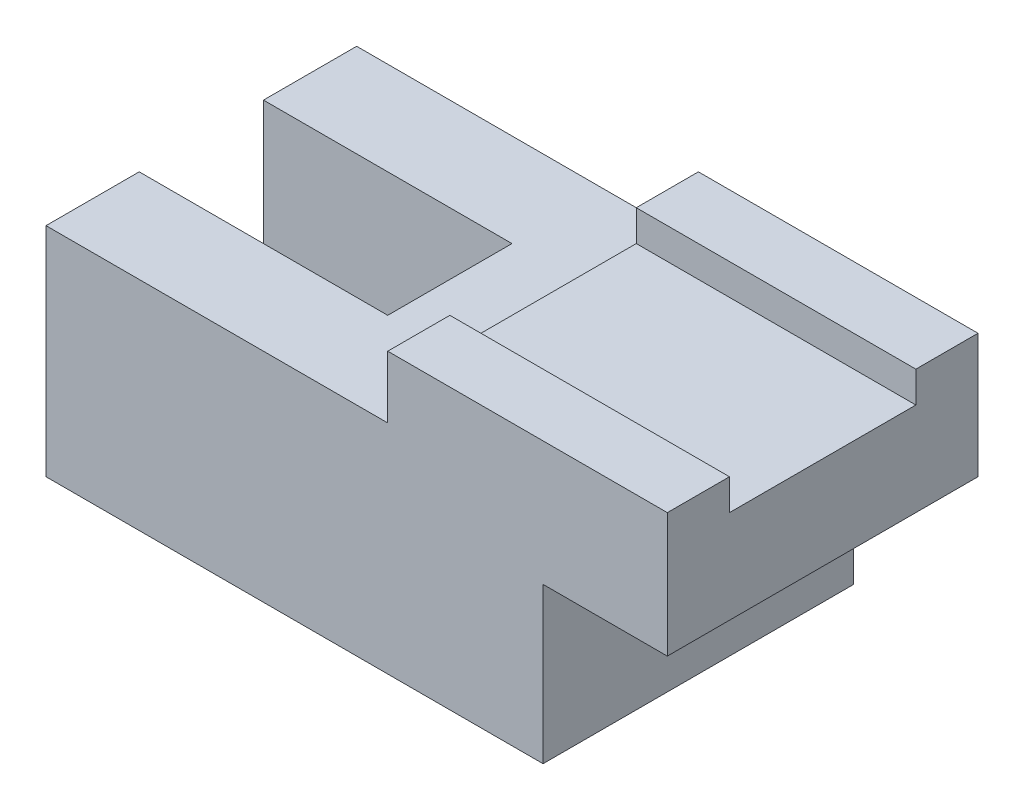
ISO-10303-21;
HEADER;
FILE_DESCRIPTION(('STEP AP214'),'2;1');
FILE_NAME('part.step','',(''),(''),'','','');
FILE_SCHEMA(('AUTOMOTIVE_DESIGN { 1 0 10303 214 1 1 1 1 }'));
ENDSEC;
DATA;
#1=APPLICATION_CONTEXT('core data for automotive mechanical design processes');
#2=APPLICATION_PROTOCOL_DEFINITION('international standard','automotive_design',2000,#1);
#3=PRODUCT_CONTEXT('',#1,'mechanical');
#4=PRODUCT('Part','Part','',(#3));
#5=PRODUCT_RELATED_PRODUCT_CATEGORY('part','',(#4));
#6=PRODUCT_DEFINITION_FORMATION('','',#4);
#7=PRODUCT_DEFINITION_CONTEXT('part definition',#1,'design');
#8=PRODUCT_DEFINITION('design','',#6,#7);
#9=PRODUCT_DEFINITION_SHAPE('','',#8);
#10=(LENGTH_UNIT() NAMED_UNIT(*) SI_UNIT(.MILLI.,.METRE.));
#11=(NAMED_UNIT(*) PLANE_ANGLE_UNIT() SI_UNIT($,.RADIAN.));
#12=(NAMED_UNIT(*) SI_UNIT($,.STERADIAN.) SOLID_ANGLE_UNIT());
#13=UNCERTAINTY_MEASURE_WITH_UNIT(LENGTH_MEASURE(1.E-05),#10,'distance_accuracy_value','');
#14=(GEOMETRIC_REPRESENTATION_CONTEXT(3) GLOBAL_UNCERTAINTY_ASSIGNED_CONTEXT((#13)) GLOBAL_UNIT_ASSIGNED_CONTEXT((#10,
#11,#12)) REPRESENTATION_CONTEXT('',''));
#15=CARTESIAN_POINT('',(0.,0.,0.));
#16=DIRECTION('',(0.,0.,1.));
#17=DIRECTION('',(1.,0.,0.));
#18=AXIS2_PLACEMENT_3D('',#15,#16,#17);
#19=CARTESIAN_POINT('',(100.,45.,50.));
#20=DIRECTION('',(0.,-1.,0.));
#21=DIRECTION('',(1.,0.,0.));
#22=AXIS2_PLACEMENT_3D('',#19,#20,#21);
#23=PLANE('',#22);
#24=DIRECTION('',(0.,0.,-1.));
#25=VECTOR('',#24,1.);
#26=CARTESIAN_POINT('',(100.,45.,50.));
#27=LINE('',#26,#25);
#28=CARTESIAN_POINT('',(100.,45.,50.));
#29=VERTEX_POINT('',#28);
#30=CARTESIAN_POINT('',(100.,45.,40.));
#31=VERTEX_POINT('',#30);
#32=EDGE_CURVE('E171',#29,#31,#27,.T.);
#33=ORIENTED_EDGE('',*,*,#32,.T.);
#34=DIRECTION('',(-1.,0.,0.));
#35=VECTOR('',#34,1.);
#36=CARTESIAN_POINT('',(100.,45.,40.));
#37=LINE('',#36,#35);
#38=CARTESIAN_POINT('',(55.,45.,40.));
#39=VERTEX_POINT('',#38);
#40=EDGE_CURVE('E279',#31,#39,#37,.T.);
#41=ORIENTED_EDGE('',*,*,#40,.T.);
#42=DIRECTION('',(0.,0.,-1.));
#43=VECTOR('',#42,1.);
#44=CARTESIAN_POINT('',(55.,45.,50.));
#45=LINE('',#44,#43);
#46=CARTESIAN_POINT('',(55.,45.,50.));
#47=VERTEX_POINT('',#46);
#48=EDGE_CURVE('E178',#47,#39,#45,.T.);
#49=ORIENTED_EDGE('',*,*,#48,.F.);
#50=DIRECTION('',(-1.,0.,0.));
#51=VECTOR('',#50,1.);
#52=CARTESIAN_POINT('',(100.,45.,50.));
#53=LINE('',#52,#51);
#54=EDGE_CURVE('E251',#29,#47,#53,.T.);
#55=ORIENTED_EDGE('',*,*,#54,.F.);
#56=EDGE_LOOP('',(#33,#41,#49,#55));
#57=FACE_BOUND('',#56,.T.);
#58=ADVANCED_FACE('F39',(#57),#23,.F.);
#59=CARTESIAN_POINT('',(0.,35.,50.));
#60=DIRECTION('',(1.,0.,0.));
#61=DIRECTION('',(0.,0.,-1.));
#62=AXIS2_PLACEMENT_3D('',#59,#60,#61);
#63=PLANE('',#62);
#64=DIRECTION('',(0.,0.,-1.));
#65=VECTOR('',#64,1.);
#66=CARTESIAN_POINT('',(0.,0.,50.));
#67=LINE('',#66,#65);
#68=CARTESIAN_POINT('',(0.,0.,15.));
#69=VERTEX_POINT('',#68);
#70=CARTESIAN_POINT('',(0.,0.,0.));
#71=VERTEX_POINT('',#70);
#72=EDGE_CURVE('E50',#69,#71,#67,.T.);
#73=ORIENTED_EDGE('',*,*,#72,.F.);
#74=DIRECTION('',(0.,-1.,0.));
#75=VECTOR('',#74,1.);
#76=CARTESIAN_POINT('',(0.,0.,15.));
#77=LINE('',#76,#75);
#78=CARTESIAN_POINT('',(0.,35.,15.));
#79=VERTEX_POINT('',#78);
#80=EDGE_CURVE('E272',#79,#69,#77,.T.);
#81=ORIENTED_EDGE('',*,*,#80,.F.);
#82=DIRECTION('',(0.,0.,-1.));
#83=VECTOR('',#82,1.);
#84=CARTESIAN_POINT('',(0.,35.,50.));
#85=LINE('',#84,#83);
#86=CARTESIAN_POINT('',(0.,35.,0.));
#87=VERTEX_POINT('',#86);
#88=EDGE_CURVE('E212',#79,#87,#85,.T.);
#89=ORIENTED_EDGE('',*,*,#88,.T.);
#90=DIRECTION('',(0.,-1.,0.));
#91=VECTOR('',#90,1.);
#92=CARTESIAN_POINT('',(0.,35.,0.));
#93=LINE('',#92,#91);
#94=EDGE_CURVE('E208',#87,#71,#93,.T.);
#95=ORIENTED_EDGE('',*,*,#94,.T.);
#96=EDGE_LOOP('',(#73,#81,#89,#95));
#97=FACE_BOUND('',#96,.T.);
#98=ADVANCED_FACE('F215',(#97),#63,.F.);
#99=CARTESIAN_POINT('',(0.,35.,50.));
#100=VERTEX_POINT('',#99);
#101=CARTESIAN_POINT('',(0.,35.,35.));
#102=VERTEX_POINT('',#101);
#103=EDGE_CURVE('E234',#100,#102,#85,.T.);
#104=ORIENTED_EDGE('',*,*,#103,.T.);
#105=DIRECTION('',(0.,1.,0.));
#106=VECTOR('',#105,1.);
#107=CARTESIAN_POINT('',(0.,35.,35.));
#108=LINE('',#107,#106);
#109=CARTESIAN_POINT('',(0.,0.,35.));
#110=VERTEX_POINT('',#109);
#111=EDGE_CURVE('E277',#110,#102,#108,.T.);
#112=ORIENTED_EDGE('',*,*,#111,.F.);
#113=CARTESIAN_POINT('',(0.,0.,50.));
#114=VERTEX_POINT('',#113);
#115=EDGE_CURVE('E11',#114,#110,#67,.T.);
#116=ORIENTED_EDGE('',*,*,#115,.F.);
#117=DIRECTION('',(0.,-1.,0.));
#118=VECTOR('',#117,1.);
#119=CARTESIAN_POINT('',(0.,35.,50.));
#120=LINE('',#119,#118);
#121=EDGE_CURVE('E231',#100,#114,#120,.T.);
#122=ORIENTED_EDGE('',*,*,#121,.F.);
#123=EDGE_LOOP('',(#104,#112,#116,#122));
#124=FACE_BOUND('',#123,.T.);
#125=ADVANCED_FACE('F41',(#124),#63,.F.);
#126=CARTESIAN_POINT('',(0.,0.,50.));
#127=DIRECTION('',(0.,1.,0.));
#128=DIRECTION('',(0.,0.,1.));
#129=AXIS2_PLACEMENT_3D('',#126,#127,#128);
#130=PLANE('',#129);
#131=DIRECTION('',(0.,0.,1.));
#132=VECTOR('',#131,1.);
#133=CARTESIAN_POINT('',(40.,0.,35.));
#134=LINE('',#133,#132);
#135=CARTESIAN_POINT('',(40.,0.,15.));
#136=VERTEX_POINT('',#135);
#137=CARTESIAN_POINT('',(40.,0.,35.));
#138=VERTEX_POINT('',#137);
#139=EDGE_CURVE('E274',#136,#138,#134,.T.);
#140=ORIENTED_EDGE('',*,*,#139,.F.);
#141=DIRECTION('',(-1.,0.,0.));
#142=VECTOR('',#141,1.);
#143=CARTESIAN_POINT('',(40.,0.,15.));
#144=LINE('',#143,#142);
#145=EDGE_CURVE('E199',#136,#69,#144,.T.);
#146=ORIENTED_EDGE('',*,*,#145,.T.);
#147=ORIENTED_EDGE('',*,*,#72,.T.);
#148=DIRECTION('',(1.,0.,0.));
#149=VECTOR('',#148,1.);
#150=CARTESIAN_POINT('',(0.,0.,0.));
#151=LINE('',#150,#149);
#152=CARTESIAN_POINT('',(80.,0.,0.));
#153=VERTEX_POINT('',#152);
#154=EDGE_CURVE('E200',#71,#153,#151,.T.);
#155=ORIENTED_EDGE('',*,*,#154,.T.);
#156=DIRECTION('',(0.,0.,-1.));
#157=VECTOR('',#156,1.);
#158=CARTESIAN_POINT('',(80.,0.,50.));
#159=LINE('',#158,#157);
#160=CARTESIAN_POINT('',(80.,0.,50.));
#161=VERTEX_POINT('',#160);
#162=EDGE_CURVE('E189',#161,#153,#159,.T.);
#163=ORIENTED_EDGE('',*,*,#162,.F.);
#164=DIRECTION('',(1.,0.,0.));
#165=VECTOR('',#164,1.);
#166=CARTESIAN_POINT('',(0.,0.,50.));
#167=LINE('',#166,#165);
#168=EDGE_CURVE('E263',#114,#161,#167,.T.);
#169=ORIENTED_EDGE('',*,*,#168,.F.);
#170=ORIENTED_EDGE('',*,*,#115,.T.);
#171=DIRECTION('',(-1.,0.,0.));
#172=VECTOR('',#171,1.);
#173=CARTESIAN_POINT('',(40.,0.,35.));
#174=LINE('',#173,#172);
#175=EDGE_CURVE('E266',#138,#110,#174,.T.);
#176=ORIENTED_EDGE('',*,*,#175,.F.);
#177=EDGE_LOOP('',(#140,#146,#147,#155,#163,#169,#170,#176));
#178=FACE_BOUND('',#177,.T.);
#179=ADVANCED_FACE('F196',(#178),#130,.F.);
#180=CARTESIAN_POINT('',(80.,0.,50.));
#181=DIRECTION('',(-1.,0.,0.));
#182=DIRECTION('',(0.,0.,1.));
#183=AXIS2_PLACEMENT_3D('',#180,#181,#182);
#184=PLANE('',#183);
#185=DIRECTION('',(0.,1.,0.));
#186=VECTOR('',#185,1.);
#187=CARTESIAN_POINT('',(80.,0.,0.));
#188=LINE('',#187,#186);
#189=CARTESIAN_POINT('',(80.,25.,0.));
#190=VERTEX_POINT('',#189);
#191=EDGE_CURVE('E209',#153,#190,#188,.T.);
#192=ORIENTED_EDGE('',*,*,#191,.T.);
#193=DIRECTION('',(0.,0.,-1.));
#194=VECTOR('',#193,1.);
#195=CARTESIAN_POINT('',(80.,25.,50.));
#196=LINE('',#195,#194);
#197=CARTESIAN_POINT('',(80.,25.,50.));
#198=VERTEX_POINT('',#197);
#199=EDGE_CURVE('E183',#198,#190,#196,.T.);
#200=ORIENTED_EDGE('',*,*,#199,.F.);
#201=DIRECTION('',(0.,1.,0.));
#202=VECTOR('',#201,1.);
#203=CARTESIAN_POINT('',(80.,0.,50.));
#204=LINE('',#203,#202);
#205=EDGE_CURVE('E261',#161,#198,#204,.T.);
#206=ORIENTED_EDGE('',*,*,#205,.F.);
#207=ORIENTED_EDGE('',*,*,#162,.T.);
#208=EDGE_LOOP('',(#192,#200,#206,#207));
#209=FACE_BOUND('',#208,.T.);
#210=ADVANCED_FACE('F311',(#209),#184,.F.);
#211=CARTESIAN_POINT('',(80.,25.,50.));
#212=DIRECTION('',(0.,1.,0.));
#213=DIRECTION('',(0.,0.,1.));
#214=AXIS2_PLACEMENT_3D('',#211,#212,#213);
#215=PLANE('',#214);
#216=DIRECTION('',(1.,0.,0.));
#217=VECTOR('',#216,1.);
#218=CARTESIAN_POINT('',(80.,25.,0.));
#219=LINE('',#218,#217);
#220=CARTESIAN_POINT('',(100.,25.,0.));
#221=VERTEX_POINT('',#220);
#222=EDGE_CURVE('E221',#190,#221,#219,.T.);
#223=ORIENTED_EDGE('',*,*,#222,.T.);
#224=DIRECTION('',(0.,0.,-1.));
#225=VECTOR('',#224,1.);
#226=CARTESIAN_POINT('',(100.,25.,50.));
#227=LINE('',#226,#225);
#228=CARTESIAN_POINT('',(100.,25.,50.));
#229=VERTEX_POINT('',#228);
#230=EDGE_CURVE('E179',#229,#221,#227,.T.);
#231=ORIENTED_EDGE('',*,*,#230,.F.);
#232=DIRECTION('',(1.,0.,0.));
#233=VECTOR('',#232,1.);
#234=CARTESIAN_POINT('',(80.,25.,50.));
#235=LINE('',#234,#233);
#236=EDGE_CURVE('E259',#198,#229,#235,.T.);
#237=ORIENTED_EDGE('',*,*,#236,.F.);
#238=ORIENTED_EDGE('',*,*,#199,.T.);
#239=EDGE_LOOP('',(#223,#231,#237,#238));
#240=FACE_BOUND('',#239,.T.);
#241=ADVANCED_FACE('F320',(#240),#215,.F.);
#242=CARTESIAN_POINT('',(100.,25.,50.));
#243=DIRECTION('',(-1.,0.,0.));
#244=DIRECTION('',(0.,0.,1.));
#245=AXIS2_PLACEMENT_3D('',#242,#243,#244);
#246=PLANE('',#245);
#247=DIRECTION('',(0.,0.,1.));
#248=VECTOR('',#247,1.);
#249=CARTESIAN_POINT('',(100.,40.,10.));
#250=LINE('',#249,#248);
#251=CARTESIAN_POINT('',(100.,40.,10.));
#252=VERTEX_POINT('',#251);
#253=CARTESIAN_POINT('',(100.,40.,40.));
#254=VERTEX_POINT('',#253);
#255=EDGE_CURVE('E158',#252,#254,#250,.T.);
#256=ORIENTED_EDGE('',*,*,#255,.T.);
#257=DIRECTION('',(0.,1.,0.));
#258=VECTOR('',#257,1.);
#259=CARTESIAN_POINT('',(100.,40.,40.));
#260=LINE('',#259,#258);
#261=EDGE_CURVE('E169',#254,#31,#260,.T.);
#262=ORIENTED_EDGE('',*,*,#261,.T.);
#263=ORIENTED_EDGE('',*,*,#32,.F.);
#264=DIRECTION('',(0.,1.,0.));
#265=VECTOR('',#264,1.);
#266=CARTESIAN_POINT('',(100.,25.,50.));
#267=LINE('',#266,#265);
#268=EDGE_CURVE('E254',#229,#29,#267,.T.);
#269=ORIENTED_EDGE('',*,*,#268,.F.);
#270=ORIENTED_EDGE('',*,*,#230,.T.);
#271=DIRECTION('',(0.,1.,0.));
#272=VECTOR('',#271,1.);
#273=CARTESIAN_POINT('',(100.,25.,0.));
#274=LINE('',#273,#272);
#275=CARTESIAN_POINT('',(100.,45.,0.));
#276=VERTEX_POINT('',#275);
#277=EDGE_CURVE('E172',#221,#276,#274,.T.);
#278=ORIENTED_EDGE('',*,*,#277,.T.);
#279=CARTESIAN_POINT('',(100.,45.,10.));
#280=VERTEX_POINT('',#279);
#281=EDGE_CURVE('E164',#280,#276,#27,.T.);
#282=ORIENTED_EDGE('',*,*,#281,.F.);
#283=DIRECTION('',(0.,-1.,0.));
#284=VECTOR('',#283,1.);
#285=CARTESIAN_POINT('',(100.,45.,10.));
#286=LINE('',#285,#284);
#287=EDGE_CURVE('E151',#280,#252,#286,.T.);
#288=ORIENTED_EDGE('',*,*,#287,.T.);
#289=EDGE_LOOP('',(#256,#262,#263,#269,#270,#278,#282,#288));
#290=FACE_BOUND('',#289,.T.);
#291=ADVANCED_FACE('F168',(#290),#246,.F.);
#292=CARTESIAN_POINT('',(55.,45.,10.));
#293=VERTEX_POINT('',#292);
#294=CARTESIAN_POINT('',(55.,45.,0.));
#295=VERTEX_POINT('',#294);
#296=EDGE_CURVE('E170',#293,#295,#45,.T.);
#297=ORIENTED_EDGE('',*,*,#296,.F.);
#298=DIRECTION('',(-1.,0.,0.));
#299=VECTOR('',#298,1.);
#300=CARTESIAN_POINT('',(100.,45.,10.));
#301=LINE('',#300,#299);
#302=EDGE_CURVE('E53',#280,#293,#301,.T.);
#303=ORIENTED_EDGE('',*,*,#302,.F.);
#304=ORIENTED_EDGE('',*,*,#281,.T.);
#305=DIRECTION('',(-1.,0.,0.));
#306=VECTOR('',#305,1.);
#307=CARTESIAN_POINT('',(100.,45.,0.));
#308=LINE('',#307,#306);
#309=EDGE_CURVE('E229',#276,#295,#308,.T.);
#310=ORIENTED_EDGE('',*,*,#309,.T.);
#311=EDGE_LOOP('',(#297,#303,#304,#310));
#312=FACE_BOUND('',#311,.T.);
#313=ADVANCED_FACE('F162',(#312),#23,.F.);
#314=CARTESIAN_POINT('',(55.,45.,50.));
#315=DIRECTION('',(1.,0.,0.));
#316=DIRECTION('',(0.,1.,0.));
#317=AXIS2_PLACEMENT_3D('',#314,#315,#316);
#318=PLANE('',#317);
#319=ORIENTED_EDGE('',*,*,#48,.T.);
#320=DIRECTION('',(0.,1.,0.));
#321=VECTOR('',#320,1.);
#322=CARTESIAN_POINT('',(55.,40.,40.));
#323=LINE('',#322,#321);
#324=CARTESIAN_POINT('',(55.,40.,40.));
#325=VERTEX_POINT('',#324);
#326=EDGE_CURVE('E157',#325,#39,#323,.T.);
#327=ORIENTED_EDGE('',*,*,#326,.F.);
#328=DIRECTION('',(0.,0.,1.));
#329=VECTOR('',#328,1.);
#330=CARTESIAN_POINT('',(55.,40.,10.));
#331=LINE('',#330,#329);
#332=CARTESIAN_POINT('',(55.,40.,10.));
#333=VERTEX_POINT('',#332);
#334=EDGE_CURVE('E292',#333,#325,#331,.T.);
#335=ORIENTED_EDGE('',*,*,#334,.F.);
#336=DIRECTION('',(0.,-1.,0.));
#337=VECTOR('',#336,1.);
#338=CARTESIAN_POINT('',(55.,45.,10.));
#339=LINE('',#338,#337);
#340=EDGE_CURVE('E241',#293,#333,#339,.T.);
#341=ORIENTED_EDGE('',*,*,#340,.F.);
#342=ORIENTED_EDGE('',*,*,#296,.T.);
#343=DIRECTION('',(0.,-1.,0.));
#344=VECTOR('',#343,1.);
#345=CARTESIAN_POINT('',(55.,45.,0.));
#346=LINE('',#345,#344);
#347=CARTESIAN_POINT('',(55.,35.,0.));
#348=VERTEX_POINT('',#347);
#349=EDGE_CURVE('E230',#295,#348,#346,.T.);
#350=ORIENTED_EDGE('',*,*,#349,.T.);
#351=DIRECTION('',(0.,0.,-1.));
#352=VECTOR('',#351,1.);
#353=CARTESIAN_POINT('',(55.,35.,50.));
#354=LINE('',#353,#352);
#355=CARTESIAN_POINT('',(55.,35.,50.));
#356=VERTEX_POINT('',#355);
#357=EDGE_CURVE('E237',#356,#348,#354,.T.);
#358=ORIENTED_EDGE('',*,*,#357,.F.);
#359=DIRECTION('',(0.,-1.,0.));
#360=VECTOR('',#359,1.);
#361=CARTESIAN_POINT('',(55.,45.,50.));
#362=LINE('',#361,#360);
#363=EDGE_CURVE('E249',#47,#356,#362,.T.);
#364=ORIENTED_EDGE('',*,*,#363,.F.);
#365=EDGE_LOOP('',(#319,#327,#335,#341,#342,#350,#358,#364));
#366=FACE_BOUND('',#365,.T.);
#367=ADVANCED_FACE('F244',(#366),#318,.F.);
#368=CARTESIAN_POINT('',(55.,35.,50.));
#369=DIRECTION('',(0.,-1.,0.));
#370=DIRECTION('',(1.,0.,0.));
#371=AXIS2_PLACEMENT_3D('',#368,#369,#370);
#372=PLANE('',#371);
#373=ORIENTED_EDGE('',*,*,#88,.F.);
#374=DIRECTION('',(-1.,0.,0.));
#375=VECTOR('',#374,1.);
#376=CARTESIAN_POINT('',(40.,35.,15.));
#377=LINE('',#376,#375);
#378=CARTESIAN_POINT('',(40.,35.,15.));
#379=VERTEX_POINT('',#378);
#380=EDGE_CURVE('E220',#379,#79,#377,.T.);
#381=ORIENTED_EDGE('',*,*,#380,.F.);
#382=DIRECTION('',(0.,0.,-1.));
#383=VECTOR('',#382,1.);
#384=CARTESIAN_POINT('',(40.,35.,15.));
#385=LINE('',#384,#383);
#386=CARTESIAN_POINT('',(40.,35.,35.));
#387=VERTEX_POINT('',#386);
#388=EDGE_CURVE('E283',#387,#379,#385,.T.);
#389=ORIENTED_EDGE('',*,*,#388,.F.);
#390=DIRECTION('',(-1.,0.,0.));
#391=VECTOR('',#390,1.);
#392=CARTESIAN_POINT('',(40.,35.,35.));
#393=LINE('',#392,#391);
#394=EDGE_CURVE('E268',#387,#102,#393,.T.);
#395=ORIENTED_EDGE('',*,*,#394,.T.);
#396=ORIENTED_EDGE('',*,*,#103,.F.);
#397=DIRECTION('',(-1.,0.,0.));
#398=VECTOR('',#397,1.);
#399=CARTESIAN_POINT('',(55.,35.,50.));
#400=LINE('',#399,#398);
#401=EDGE_CURVE('E219',#356,#100,#400,.T.);
#402=ORIENTED_EDGE('',*,*,#401,.F.);
#403=ORIENTED_EDGE('',*,*,#357,.T.);
#404=DIRECTION('',(-1.,0.,0.));
#405=VECTOR('',#404,1.);
#406=CARTESIAN_POINT('',(55.,35.,0.));
#407=LINE('',#406,#405);
#408=EDGE_CURVE('E233',#348,#87,#407,.T.);
#409=ORIENTED_EDGE('',*,*,#408,.T.);
#410=EDGE_LOOP('',(#373,#381,#389,#395,#396,#402,#403,#409));
#411=FACE_BOUND('',#410,.T.);
#412=ADVANCED_FACE('F248',(#411),#372,.F.);
#413=CARTESIAN_POINT('',(0.,0.,50.));
#414=DIRECTION('',(0.,0.,1.));
#415=DIRECTION('',(1.,0.,0.));
#416=AXIS2_PLACEMENT_3D('',#413,#414,#415);
#417=PLANE('',#416);
#418=ORIENTED_EDGE('',*,*,#121,.T.);
#419=ORIENTED_EDGE('',*,*,#168,.T.);
#420=ORIENTED_EDGE('',*,*,#205,.T.);
#421=ORIENTED_EDGE('',*,*,#236,.T.);
#422=ORIENTED_EDGE('',*,*,#268,.T.);
#423=ORIENTED_EDGE('',*,*,#54,.T.);
#424=ORIENTED_EDGE('',*,*,#363,.T.);
#425=ORIENTED_EDGE('',*,*,#401,.T.);
#426=EDGE_LOOP('',(#418,#419,#420,#421,#422,#423,#424,#425));
#427=FACE_BOUND('',#426,.T.);
#428=ADVANCED_FACE('F313',(#427),#417,.T.);
#429=CARTESIAN_POINT('',(0.,0.,0.));
#430=DIRECTION('',(0.,0.,1.));
#431=DIRECTION('',(1.,0.,0.));
#432=AXIS2_PLACEMENT_3D('',#429,#430,#431);
#433=PLANE('',#432);
#434=ORIENTED_EDGE('',*,*,#94,.F.);
#435=ORIENTED_EDGE('',*,*,#408,.F.);
#436=ORIENTED_EDGE('',*,*,#349,.F.);
#437=ORIENTED_EDGE('',*,*,#309,.F.);
#438=ORIENTED_EDGE('',*,*,#277,.F.);
#439=ORIENTED_EDGE('',*,*,#222,.F.);
#440=ORIENTED_EDGE('',*,*,#191,.F.);
#441=ORIENTED_EDGE('',*,*,#154,.F.);
#442=EDGE_LOOP('',(#434,#435,#436,#437,#438,#439,#440,#441));
#443=FACE_BOUND('',#442,.T.);
#444=ADVANCED_FACE('F206',(#443),#433,.F.);
#445=CARTESIAN_POINT('',(40.,0.,15.));
#446=DIRECTION('',(0.,0.,-1.));
#447=DIRECTION('',(-1.,0.,0.));
#448=AXIS2_PLACEMENT_3D('',#445,#446,#447);
#449=PLANE('',#448);
#450=ORIENTED_EDGE('',*,*,#80,.T.);
#451=ORIENTED_EDGE('',*,*,#145,.F.);
#452=DIRECTION('',(0.,-1.,0.));
#453=VECTOR('',#452,1.);
#454=CARTESIAN_POINT('',(40.,0.,15.));
#455=LINE('',#454,#453);
#456=EDGE_CURVE('E267',#379,#136,#455,.T.);
#457=ORIENTED_EDGE('',*,*,#456,.F.);
#458=ORIENTED_EDGE('',*,*,#380,.T.);
#459=EDGE_LOOP('',(#450,#451,#457,#458));
#460=FACE_BOUND('',#459,.T.);
#461=ADVANCED_FACE('F350',(#460),#449,.F.);
#462=CARTESIAN_POINT('',(40.,35.,35.));
#463=DIRECTION('',(0.,0.,1.));
#464=DIRECTION('',(1.,0.,0.));
#465=AXIS2_PLACEMENT_3D('',#462,#463,#464);
#466=PLANE('',#465);
#467=ORIENTED_EDGE('',*,*,#111,.T.);
#468=ORIENTED_EDGE('',*,*,#394,.F.);
#469=DIRECTION('',(0.,1.,0.));
#470=VECTOR('',#469,1.);
#471=CARTESIAN_POINT('',(40.,35.,35.));
#472=LINE('',#471,#470);
#473=EDGE_CURVE('E64',#138,#387,#472,.T.);
#474=ORIENTED_EDGE('',*,*,#473,.F.);
#475=ORIENTED_EDGE('',*,*,#175,.T.);
#476=EDGE_LOOP('',(#467,#468,#474,#475));
#477=FACE_BOUND('',#476,.T.);
#478=ADVANCED_FACE('F349',(#477),#466,.F.);
#479=CARTESIAN_POINT('',(40.,0.,0.));
#480=DIRECTION('',(1.,0.,0.));
#481=DIRECTION('',(0.,0.,-1.));
#482=AXIS2_PLACEMENT_3D('',#479,#480,#481);
#483=PLANE('',#482);
#484=ORIENTED_EDGE('',*,*,#139,.T.);
#485=ORIENTED_EDGE('',*,*,#473,.T.);
#486=ORIENTED_EDGE('',*,*,#388,.T.);
#487=ORIENTED_EDGE('',*,*,#456,.T.);
#488=EDGE_LOOP('',(#484,#485,#486,#487));
#489=FACE_BOUND('',#488,.T.);
#490=ADVANCED_FACE('F354',(#489),#483,.F.);
#491=CARTESIAN_POINT('',(100.,40.,40.));
#492=DIRECTION('',(0.,0.,1.));
#493=DIRECTION('',(1.,0.,0.));
#494=AXIS2_PLACEMENT_3D('',#491,#492,#493);
#495=PLANE('',#494);
#496=ORIENTED_EDGE('',*,*,#326,.T.);
#497=ORIENTED_EDGE('',*,*,#40,.F.);
#498=ORIENTED_EDGE('',*,*,#261,.F.);
#499=DIRECTION('',(-1.,0.,0.));
#500=VECTOR('',#499,1.);
#501=CARTESIAN_POINT('',(100.,40.,40.));
#502=LINE('',#501,#500);
#503=EDGE_CURVE('E288',#254,#325,#502,.T.);
#504=ORIENTED_EDGE('',*,*,#503,.T.);
#505=EDGE_LOOP('',(#496,#497,#498,#504));
#506=FACE_BOUND('',#505,.T.);
#507=ADVANCED_FACE('F301',(#506),#495,.F.);
#508=CARTESIAN_POINT('',(100.,40.,10.));
#509=DIRECTION('',(0.,-1.,0.));
#510=DIRECTION('',(1.,0.,0.));
#511=AXIS2_PLACEMENT_3D('',#508,#509,#510);
#512=PLANE('',#511);
#513=ORIENTED_EDGE('',*,*,#334,.T.);
#514=ORIENTED_EDGE('',*,*,#503,.F.);
#515=ORIENTED_EDGE('',*,*,#255,.F.);
#516=DIRECTION('',(-1.,0.,0.));
#517=VECTOR('',#516,1.);
#518=CARTESIAN_POINT('',(100.,40.,10.));
#519=LINE('',#518,#517);
#520=EDGE_CURVE('E153',#252,#333,#519,.T.);
#521=ORIENTED_EDGE('',*,*,#520,.T.);
#522=EDGE_LOOP('',(#513,#514,#515,#521));
#523=FACE_BOUND('',#522,.T.);
#524=ADVANCED_FACE('F296',(#523),#512,.F.);
#525=CARTESIAN_POINT('',(100.,45.,10.));
#526=DIRECTION('',(0.,0.,-1.));
#527=DIRECTION('',(-1.,0.,0.));
#528=AXIS2_PLACEMENT_3D('',#525,#526,#527);
#529=PLANE('',#528);
#530=ORIENTED_EDGE('',*,*,#340,.T.);
#531=ORIENTED_EDGE('',*,*,#520,.F.);
#532=ORIENTED_EDGE('',*,*,#287,.F.);
#533=ORIENTED_EDGE('',*,*,#302,.T.);
#534=EDGE_LOOP('',(#530,#531,#532,#533));
#535=FACE_BOUND('',#534,.T.);
#536=ADVANCED_FACE('F155',(#535),#529,.F.);
#537=CLOSED_SHELL('',(#58,#98,#125,#179,#210,#241,#291,#313,#367,#412,#428,#444,#461,#478,#490,
#507,#524,#536));
#538=MANIFOLD_SOLID_BREP('B2',#537);
#539=ADVANCED_BREP_SHAPE_REPRESENTATION('',(#18,#538),#14);
#540=SHAPE_DEFINITION_REPRESENTATION(#9,#539);
ENDSEC;
END-ISO-10303-21;
